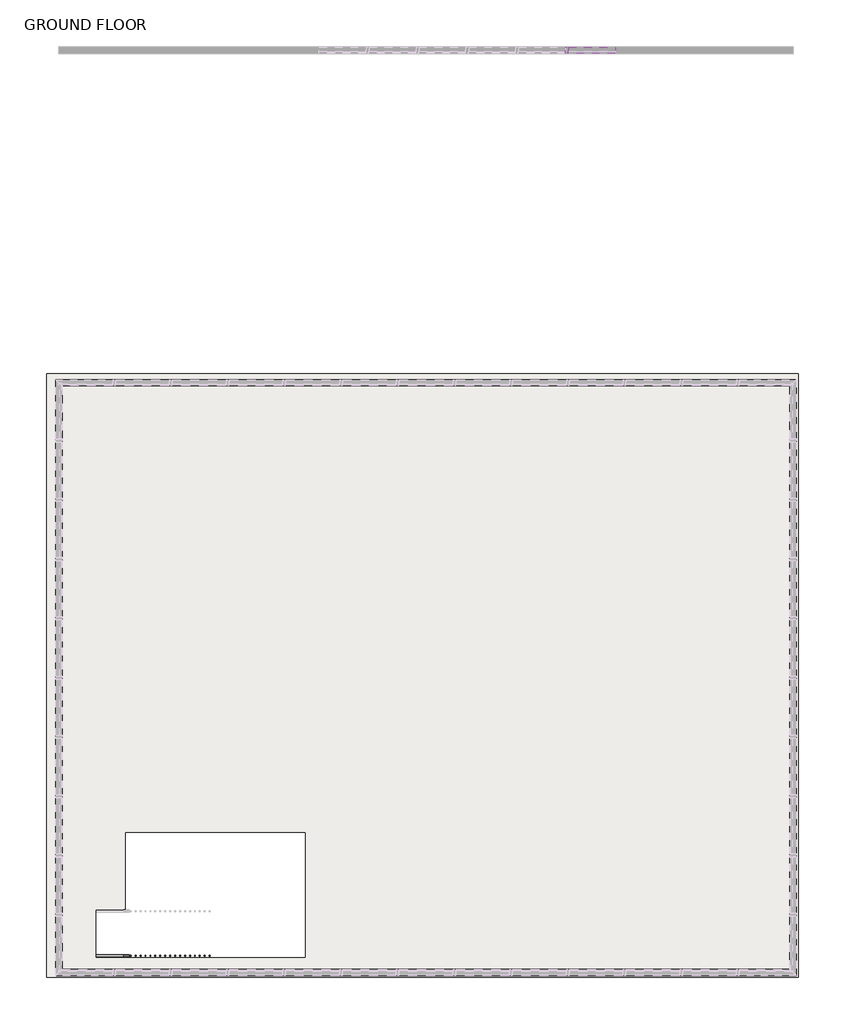
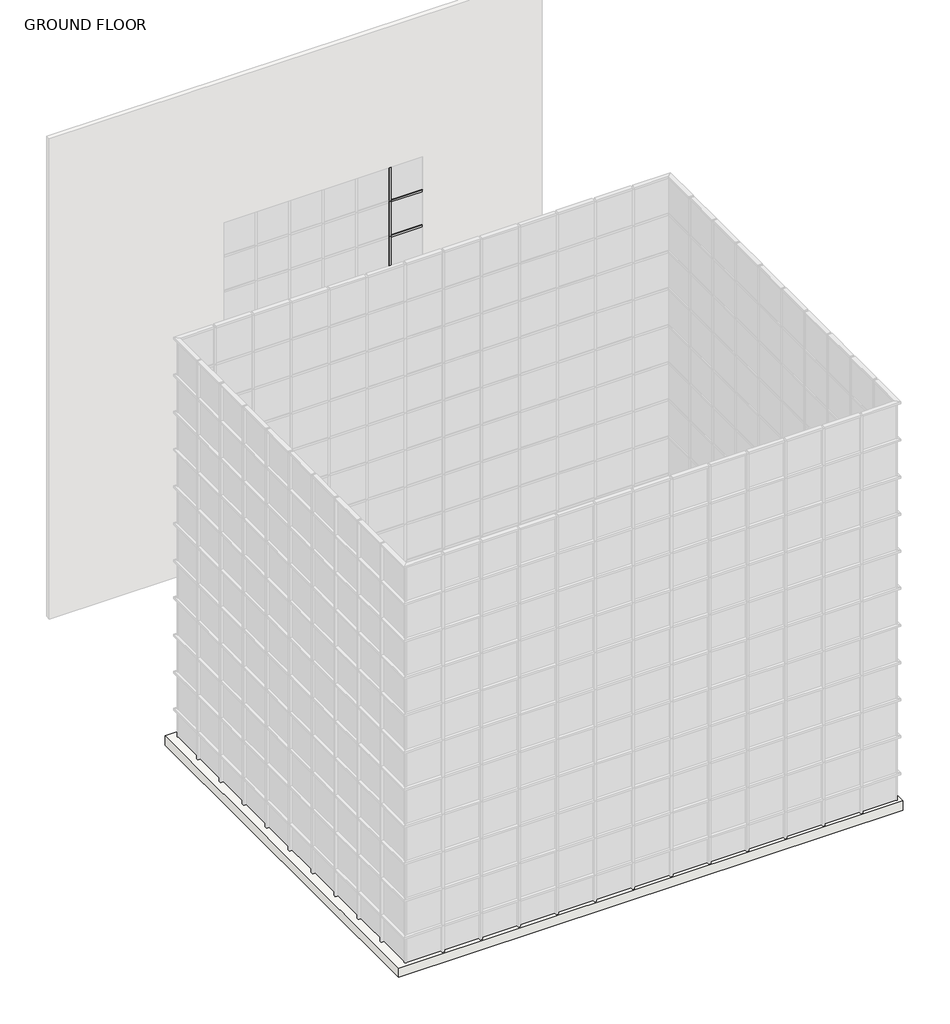
# One storey, part 15 of 16: 15 members, 1 railing, 1 slab.
"""IFC4 building model written with IfcOpenShell, lengths in millimetres."""

from ifc_helpers import new_model, si_unit, frame, origin, origin_with_axes, place, context, project, spatial, polyline, outline, extrude, faceted_brep, transform, mapped, element, save
from components import member_fdbefc00, member_3df3cfcf, member_368818a6

model = new_model("IFC4")

# Units and contexts
model_context = context("Model", 3, world=origin())
ifc_project = project(units=[si_unit("LENGTHUNIT", "METRE", prefix="MILLI")], contexts=[model_context])

# Site, building, storey
site = spatial("IfcSite", under=ifc_project)
building = spatial("IfcBuilding", under=site)
storey = spatial("IfcBuildingStorey", under=building, Name="GROUND FLOOR", Elevation=0.0)

# Members
placement = place(None, origin())
member_shape = member_fdbefc00(model_context)
element("IfcMember", 1, ObjectType="Rectangular Mullion : 2.5\" x 5\" rectangular", at=placement, inside=storey, context=model_context, shape_type="MappedRepresentation", body=[
    mapped(member_shape, transform((2306.4449607, 13200.7626438, 3045.6877023), x_axis=(0.0, 0.0, 1.0), y_axis=(0.0, -1.0, 0.0), z_axis=(1.0, 0.0, 0.0))),
])
element("IfcMember", 2, ObjectType="Rectangular Mullion : 2.5\" x 5\" rectangular", at=placement, inside=storey, context=model_context, shape_type="MappedRepresentation", body=[
    mapped(member_shape, transform((2306.4449607, 13200.7626438, 4181.5290519), x_axis=(0.0, 0.0, 1.0), y_axis=(0.0, -1.0, 0.0), z_axis=(1.0, 0.0, 0.0))),
])
element("IfcMember", 3, ObjectType="Rectangular Mullion : 2.5\" x 5\" rectangular", at=placement, inside=storey, context=model_context, shape_type="MappedRepresentation", body=[
    mapped(member_shape, transform((2306.4449607, 13200.7626438, 5317.3704015), x_axis=(0.0, 0.0, 1.0), y_axis=(0.0, -1.0, 0.0), z_axis=(1.0, 0.0, 0.0))),
])
element("IfcMember", 4, ObjectType="Rectangular Mullion : 2.5\" x 5\" rectangular", at=placement, inside=storey, context=model_context, shape_type="MappedRepresentation", body=[
    mapped(member_shape, transform((2306.4449607, 13200.7626438, 6453.2117511), x_axis=(0.0, 0.0, 1.0), y_axis=(0.0, -1.0, 0.0), z_axis=(1.0, 0.0, 0.0))),
])
element("IfcMember", 5, ObjectType="Rectangular Mullion : 2.5\" x 5\" rectangular", at=placement, inside=storey, context=model_context, shape_type="MappedRepresentation", body=[
    mapped(member_shape, transform((2306.4449607, 13200.7626438, 7589.0531007), x_axis=(0.0, 0.0, 1.0), y_axis=(0.0, -1.0, 0.0), z_axis=(1.0, 0.0, 0.0))),
])
element("IfcMember", 6, ObjectType="Rectangular Mullion : 2.5\" x 5\" rectangular", at=placement, inside=storey, context=model_context, shape_type="MappedRepresentation", body=[
    mapped(member_shape, transform((2306.4449607, 13200.7626438, 8724.8944503), x_axis=(0.0, 0.0, 1.0), y_axis=(0.0, -1.0, 0.0), z_axis=(1.0, 0.0, 0.0))),
])
element("IfcMember", 7, ObjectType="Rectangular Mullion : 2.5\" x 5\" rectangular", at=placement, inside=storey, context=model_context, shape_type="MappedRepresentation", body=[
    mapped(member_shape, transform((2306.4449607, 13200.7626438, 9860.7357999), x_axis=(0.0, 0.0, 1.0), y_axis=(0.0, -1.0, 0.0), z_axis=(1.0, 0.0, 0.0))),
])
member_2_shape = member_3df3cfcf(model_context)
element("IfcMember", 8, ObjectType="Rectangular Mullion : 2.5\" x 5\" rectangular", at=placement, inside=storey, context=model_context, shape_type="MappedRepresentation", body=[
    mapped(member_2_shape, transform((1314.3014531, 13200.7626438, 1941.5963527), x_axis=(1.0, 0.0, 0.0), y_axis=(0.0, -1.0, 0.0), z_axis=(0.0, 0.0, -1.0))),
])
member_3_shape = member_368818a6(model_context)
element("IfcMember", 9, ObjectType="Rectangular Mullion : 2.5\" x 5\" rectangular", at=placement, inside=storey, context=model_context, shape_type="MappedRepresentation", body=[
    mapped(member_3_shape, transform((1314.3014531, 13200.7626438, 3045.6877023), x_axis=(1.0, 0.0, 0.0), y_axis=(0.0, -1.0, 0.0), z_axis=(0.0, 0.0, -1.0))),
])
element("IfcMember", 10, ObjectType="Rectangular Mullion : 2.5\" x 5\" rectangular", at=placement, inside=storey, context=model_context, shape_type="MappedRepresentation", body=[
    mapped(member_3_shape, transform((1314.3014531, 13200.7626438, 4181.5290519), x_axis=(1.0, 0.0, 0.0), y_axis=(0.0, -1.0, 0.0), z_axis=(0.0, 0.0, -1.0))),
])
element("IfcMember", 11, ObjectType="Rectangular Mullion : 2.5\" x 5\" rectangular", at=placement, inside=storey, context=model_context, shape_type="MappedRepresentation", body=[
    mapped(member_3_shape, transform((1314.3014531, 13200.7626438, 5317.3704015), x_axis=(1.0, 0.0, 0.0), y_axis=(0.0, -1.0, 0.0), z_axis=(0.0, 0.0, -1.0))),
])
element("IfcMember", 12, ObjectType="Rectangular Mullion : 2.5\" x 5\" rectangular", at=placement, inside=storey, context=model_context, shape_type="MappedRepresentation", body=[
    mapped(member_3_shape, transform((1314.3014531, 13200.7626438, 6453.2117511), x_axis=(1.0, 0.0, 0.0), y_axis=(0.0, -1.0, 0.0), z_axis=(0.0, 0.0, -1.0))),
])
element("IfcMember", 13, ObjectType="Rectangular Mullion : 2.5\" x 5\" rectangular", at=placement, inside=storey, context=model_context, shape_type="MappedRepresentation", body=[
    mapped(member_3_shape, transform((1314.3014531, 13200.7626438, 7589.0531007), x_axis=(1.0, 0.0, 0.0), y_axis=(0.0, -1.0, 0.0), z_axis=(0.0, 0.0, -1.0))),
])
element("IfcMember", 14, ObjectType="Rectangular Mullion : 2.5\" x 5\" rectangular", at=placement, inside=storey, context=model_context, shape_type="MappedRepresentation", body=[
    mapped(member_3_shape, transform((1314.3014531, 13200.7626438, 8724.8944503), x_axis=(1.0, 0.0, 0.0), y_axis=(0.0, -1.0, 0.0), z_axis=(0.0, 0.0, -1.0))),
])
element("IfcMember", 15, ObjectType="Rectangular Mullion : 2.5\" x 5\" rectangular", at=placement, inside=storey, context=model_context, shape_type="MappedRepresentation", body=[
    mapped(member_2_shape, transform((1314.3014531, 13200.7626438, 9860.7357999), x_axis=(1.0, 0.0, 0.0), y_axis=(0.0, -1.0, 0.0), z_axis=(0.0, 0.0, -1.0))),
])

# Railing
element("IfcRailing", 16, ObjectType="Handrail - Rectangular", at=placement, inside=storey, context=model_context, shape_type="SolidModel", body=[
    faceted_brep([(-8362.2800418, -5370.1090076, 914.4), (-8362.2800418, -5370.1090076, 857.6038734), (-8362.2800418, -5420.9090076, 857.6038734), (-8362.2800418, -5420.9090076, 914.4), (-5009.4800418, -5370.1090076, 2590.8), (-4997.4877885, -5370.1090076, 2540.0), (-4997.4877885, -5420.9090076, 2540.0), (-5009.4800418, -5420.9090076, 2590.8), (-4120.4800418, -5370.1090076, 2590.8), (-4120.4800418, -5370.1090076, 2540.0), (-4069.6800418, -5420.9090076, 2540.0), (-4069.6800418, -5420.9090076, 2590.8), (-4120.4800418, -2917.1346494, 2590.8), (-4120.4800418, -2917.1346494, 2540.0), (-4069.6800418, -2866.3346494, 2540.0), (-4069.6800418, -2866.3346494, 2590.8), (-5009.4800418, -2917.1346494, 2590.8), (-5021.472295, -2917.1346494, 2540.0), (-5021.472295, -2866.3346494, 2540.0), (-5009.4800418, -2866.3346494, 2590.8), (-7752.6800418, -2917.1346494, 3962.4), (-7752.6800418, -2866.3346494, 3962.4), (-7752.6800418, -2866.3346494, 3905.6038734), (-7752.6800418, -2917.1346494, 3905.6038734)], [[[0, 1, 2, 3]], [[1, 0, 4, 5]], [[2, 1, 5, 6]], [[3, 2, 6, 7]], [[0, 3, 7, 4]], [[5, 4, 8, 9]], [[6, 5, 9, 10]], [[7, 6, 10, 11]], [[4, 7, 11, 8]], [[9, 8, 12, 13]], [[10, 9, 13, 14]], [[11, 10, 14, 15]], [[8, 11, 15, 12]], [[13, 12, 16, 17]], [[14, 13, 17, 18]], [[15, 14, 18, 19]], [[12, 15, 19, 16]], [[20, 21, 22, 23]], [[17, 16, 20, 23]], [[18, 17, 23, 22]], [[19, 18, 22, 21]], [[16, 19, 21, 20]]]),
    extrude(outline(polyline([(3859.5663734, -7660.6050418), (3001.9625, -7660.6050418), (2992.4375, -7641.5550418), (3850.0413734, -7641.5550418), (3859.5663734, -7660.6050418)])), frame((0.0, -2901.2596494, 0.0), z_axis=(0.0, 1.0, 0.0), x_axis=(0.0, 0.0, 1.0)), (0.0, 0.0, 1.0), 19.05),
    extrude(outline(polyline([(3808.7663734, -7559.0050418), (2951.1625, -7559.0050418), (2941.6375, -7539.9550418), (3799.2413734, -7539.9550418), (3808.7663734, -7559.0050418)])), frame((0.0, -2901.2596494, 0.0), z_axis=(0.0, 1.0, 0.0), x_axis=(0.0, 0.0, 1.0)), (0.0, 0.0, 1.0), 19.05),
    extrude(outline(polyline([(3757.9663734, -7457.4050418), (2900.3625, -7457.4050418), (2890.8375, -7438.3550418), (3748.4413734, -7438.3550418), (3757.9663734, -7457.4050418)])), frame((0.0, -2901.2596494, 0.0), z_axis=(0.0, 1.0, 0.0), x_axis=(0.0, 0.0, 1.0)), (0.0, 0.0, 1.0), 19.05),
    extrude(outline(polyline([(3707.1663734, -7355.8050418), (2849.5625, -7355.8050418), (2840.0375, -7336.7550418), (3697.6413734, -7336.7550418), (3707.1663734, -7355.8050418)])), frame((0.0, -2901.2596494, 0.0), z_axis=(0.0, 1.0, 0.0), x_axis=(0.0, 0.0, 1.0)), (0.0, 0.0, 1.0), 19.05),
    extrude(outline(polyline([(3656.3663734, -7254.2050418), (2798.7625, -7254.2050418), (2789.2375, -7235.1550418), (3646.8413734, -7235.1550418), (3656.3663734, -7254.2050418)])), frame((0.0, -2901.2596494, 0.0), z_axis=(0.0, 1.0, 0.0), x_axis=(0.0, 0.0, 1.0)), (0.0, 0.0, 1.0), 19.05),
    extrude(outline(polyline([(3605.5663734, -7152.6050418), (2747.9625, -7152.6050418), (2738.4375, -7133.5550418), (3596.0413734, -7133.5550418), (3605.5663734, -7152.6050418)])), frame((0.0, -2901.2596494, 0.0), z_axis=(0.0, 1.0, 0.0), x_axis=(0.0, 0.0, 1.0)), (0.0, 0.0, 1.0), 19.05),
    extrude(outline(polyline([(3554.7663734, -7051.0050418), (2697.1625, -7051.0050418), (2687.6375, -7031.9550418), (3545.2413734, -7031.9550418), (3554.7663734, -7051.0050418)])), frame((0.0, -2901.2596494, 0.0), z_axis=(0.0, 1.0, 0.0), x_axis=(0.0, 0.0, 1.0)), (0.0, 0.0, 1.0), 19.05),
    extrude(outline(polyline([(3503.9663734, -6949.4050418), (2646.3625, -6949.4050418), (2636.8375, -6930.3550418), (3494.4413734, -6930.3550418), (3503.9663734, -6949.4050418)])), frame((0.0, -2901.2596494, 0.0), z_axis=(0.0, 1.0, 0.0), x_axis=(0.0, 0.0, 1.0)), (0.0, 0.0, 1.0), 19.05),
    extrude(outline(polyline([(3453.1663734, -6847.8050418), (2595.5625, -6847.8050418), (2586.0375, -6828.7550418), (3443.6413734, -6828.7550418), (3453.1663734, -6847.8050418)])), frame((0.0, -2901.2596494, 0.0), z_axis=(0.0, 1.0, 0.0), x_axis=(0.0, 0.0, 1.0)), (0.0, 0.0, 1.0), 19.05),
    extrude(outline(polyline([(3402.3663734, -6746.2050418), (2544.7625, -6746.2050418), (2535.2375, -6727.1550418), (3392.8413734, -6727.1550418), (3402.3663734, -6746.2050418)])), frame((0.0, -2901.2596494, 0.0), z_axis=(0.0, 1.0, 0.0), x_axis=(0.0, 0.0, 1.0)), (0.0, 0.0, 1.0), 19.05),
    extrude(outline(polyline([(3351.5663734, -6644.6050418), (2493.9625, -6644.6050418), (2484.4375, -6625.5550418), (3342.0413734, -6625.5550418), (3351.5663734, -6644.6050418)])), frame((0.0, -2901.2596494, 0.0), z_axis=(0.0, 1.0, 0.0), x_axis=(0.0, 0.0, 1.0)), (0.0, 0.0, 1.0), 19.05),
    extrude(outline(polyline([(3300.7663734, -6543.0050418), (2443.1625, -6543.0050418), (2433.6375, -6523.9550418), (3291.2413734, -6523.9550418), (3300.7663734, -6543.0050418)])), frame((0.0, -2901.2596494, 0.0), z_axis=(0.0, 1.0, 0.0), x_axis=(0.0, 0.0, 1.0)), (0.0, 0.0, 1.0), 19.05),
    extrude(outline(polyline([(3249.9663734, -6441.4050418), (2392.3625, -6441.4050418), (2382.8375, -6422.3550418), (3240.4413734, -6422.3550418), (3249.9663734, -6441.4050418)])), frame((0.0, -2901.2596494, 0.0), z_axis=(0.0, 1.0, 0.0), x_axis=(0.0, 0.0, 1.0)), (0.0, 0.0, 1.0), 19.05),
    extrude(outline(polyline([(3199.1663734, -6339.8050418), (2341.5625, -6339.8050418), (2332.0375, -6320.7550418), (3189.6413734, -6320.7550418), (3199.1663734, -6339.8050418)])), frame((0.0, -2901.2596494, 0.0), z_axis=(0.0, 1.0, 0.0), x_axis=(0.0, 0.0, 1.0)), (0.0, 0.0, 1.0), 19.05),
    extrude(outline(polyline([(3148.3663734, -6238.2050418), (2290.7625, -6238.2050418), (2281.2375, -6219.1550418), (3138.8413734, -6219.1550418), (3148.3663734, -6238.2050418)])), frame((0.0, -2901.2596494, 0.0), z_axis=(0.0, 1.0, 0.0), x_axis=(0.0, 0.0, 1.0)), (0.0, 0.0, 1.0), 19.05),
    extrude(outline(polyline([(3097.5663734, -6136.6050418), (2239.9625, -6136.6050418), (2230.4375, -6117.5550418), (3088.0413734, -6117.5550418), (3097.5663734, -6136.6050418)])), frame((0.0, -2901.2596494, 0.0), z_axis=(0.0, 1.0, 0.0), x_axis=(0.0, 0.0, 1.0)), (0.0, 0.0, 1.0), 19.05),
    extrude(outline(polyline([(3046.7663734, -6035.0050418), (2189.1625, -6035.0050418), (2179.6375, -6015.9550418), (3037.2413734, -6015.9550418), (3046.7663734, -6035.0050418)])), frame((0.0, -2901.2596494, 0.0), z_axis=(0.0, 1.0, 0.0), x_axis=(0.0, 0.0, 1.0)), (0.0, 0.0, 1.0), 19.05),
    extrude(outline(polyline([(2995.9663734, -5933.4050418), (2138.3625, -5933.4050418), (2128.8375, -5914.3550418), (2986.4413734, -5914.3550418), (2995.9663734, -5933.4050418)])), frame((0.0, -2901.2596494, 0.0), z_axis=(0.0, 1.0, 0.0), x_axis=(0.0, 0.0, 1.0)), (0.0, 0.0, 1.0), 19.05),
    extrude(outline(polyline([(2945.1663734, -5831.8050418), (2087.5625, -5831.8050418), (2078.0375, -5812.7550418), (2935.6413734, -5812.7550418), (2945.1663734, -5831.8050418)])), frame((0.0, -2901.2596494, 0.0), z_axis=(0.0, 1.0, 0.0), x_axis=(0.0, 0.0, 1.0)), (0.0, 0.0, 1.0), 19.05),
    extrude(outline(polyline([(2894.3663734, -5730.2050418), (2036.7625, -5730.2050418), (2027.2375, -5711.1550418), (2884.8413734, -5711.1550418), (2894.3663734, -5730.2050418)])), frame((0.0, -2901.2596494, 0.0), z_axis=(0.0, 1.0, 0.0), x_axis=(0.0, 0.0, 1.0)), (0.0, 0.0, 1.0), 19.05),
    extrude(outline(polyline([(2843.5663734, -5628.6050418), (1985.9625, -5628.6050418), (1976.4375, -5609.5550418), (2834.0413734, -5609.5550418), (2843.5663734, -5628.6050418)])), frame((0.0, -2901.2596494, 0.0), z_axis=(0.0, 1.0, 0.0), x_axis=(0.0, 0.0, 1.0)), (0.0, 0.0, 1.0), 19.05),
    extrude(outline(polyline([(2792.7663734, -5527.0050418), (1935.1625, -5527.0050418), (1925.6375, -5507.9550418), (2783.2413734, -5507.9550418), (2792.7663734, -5527.0050418)])), frame((0.0, -2901.2596494, 0.0), z_axis=(0.0, 1.0, 0.0), x_axis=(0.0, 0.0, 1.0)), (0.0, 0.0, 1.0), 19.05),
    extrude(outline(polyline([(2741.9663734, -5425.4050418), (1884.3625, -5425.4050418), (1874.8375, -5406.3550418), (2732.4413734, -5406.3550418), (2741.9663734, -5425.4050418)])), frame((0.0, -2901.2596494, 0.0), z_axis=(0.0, 1.0, 0.0), x_axis=(0.0, 0.0, 1.0)), (0.0, 0.0, 1.0), 19.05),
    extrude(outline(polyline([(2691.1663734, -5323.8050418), (1833.5625, -5323.8050418), (1824.0375, -5304.7550418), (2681.6413734, -5304.7550418), (2691.1663734, -5323.8050418)])), frame((0.0, -2901.2596494, 0.0), z_axis=(0.0, 1.0, 0.0), x_axis=(0.0, 0.0, 1.0)), (0.0, 0.0, 1.0), 19.05),
    extrude(outline(polyline([(2640.3663734, -5222.2050418), (1782.7625, -5222.2050418), (1773.2375, -5203.1550418), (2630.8413734, -5203.1550418), (2640.3663734, -5222.2050418)])), frame((0.0, -2901.2596494, 0.0), z_axis=(0.0, 1.0, 0.0), x_axis=(0.0, 0.0, 1.0)), (0.0, 0.0, 1.0), 19.05),
    extrude(outline(polyline([(2589.5663734, -5120.6050418), (1731.9625, -5120.6050418), (1722.4375, -5101.5550418), (2580.0413734, -5101.5550418), (2589.5663734, -5120.6050418)])), frame((0.0, -2901.2596494, 0.0), z_axis=(0.0, 1.0, 0.0), x_axis=(0.0, 0.0, 1.0)), (0.0, 0.0, 1.0), 19.05),
    extrude(outline(polyline([(-4898.3550418, -2901.2596494), (-4917.4050418, -2901.2596494), (-4917.4050418, -2882.2096494), (-4898.3550418, -2882.2096494), (-4898.3550418, -2901.2596494)])), frame((0.0, 0.0, 1676.4), z_axis=(0.0, 0.0, 1.0), x_axis=(1.0, 0.0, 0.0)), (0.0, 0.0, 1.0), 863.6),
    extrude(outline(polyline([(-4796.7550418, -2901.2596494), (-4815.8050418, -2901.2596494), (-4815.8050418, -2882.2096494), (-4796.7550418, -2882.2096494), (-4796.7550418, -2901.2596494)])), frame((0.0, 0.0, 1676.4), z_axis=(0.0, 0.0, 1.0), x_axis=(1.0, 0.0, 0.0)), (0.0, 0.0, 1.0), 863.6),
    extrude(outline(polyline([(-4695.1550418, -2901.2596494), (-4714.2050418, -2901.2596494), (-4714.2050418, -2882.2096494), (-4695.1550418, -2882.2096494), (-4695.1550418, -2901.2596494)])), frame((0.0, 0.0, 1676.4), z_axis=(0.0, 0.0, 1.0), x_axis=(1.0, 0.0, 0.0)), (0.0, 0.0, 1.0), 863.6),
    extrude(outline(polyline([(-4593.5550418, -2901.2596494), (-4612.6050418, -2901.2596494), (-4612.6050418, -2882.2096494), (-4593.5550418, -2882.2096494), (-4593.5550418, -2901.2596494)])), frame((0.0, 0.0, 1676.4), z_axis=(0.0, 0.0, 1.0), x_axis=(1.0, 0.0, 0.0)), (0.0, 0.0, 1.0), 863.6),
    extrude(outline(polyline([(-4491.9550418, -2901.2596494), (-4511.0050418, -2901.2596494), (-4511.0050418, -2882.2096494), (-4491.9550418, -2882.2096494), (-4491.9550418, -2901.2596494)])), frame((0.0, 0.0, 1676.4), z_axis=(0.0, 0.0, 1.0), x_axis=(1.0, 0.0, 0.0)), (0.0, 0.0, 1.0), 863.6),
    extrude(outline(polyline([(-4390.3550418, -2901.2596494), (-4409.4050418, -2901.2596494), (-4409.4050418, -2882.2096494), (-4390.3550418, -2882.2096494), (-4390.3550418, -2901.2596494)])), frame((0.0, 0.0, 1676.4), z_axis=(0.0, 0.0, 1.0), x_axis=(1.0, 0.0, 0.0)), (0.0, 0.0, 1.0), 863.6),
    extrude(outline(polyline([(-4288.7550418, -2901.2596494), (-4307.8050418, -2901.2596494), (-4307.8050418, -2882.2096494), (-4288.7550418, -2882.2096494), (-4288.7550418, -2901.2596494)])), frame((0.0, 0.0, 1676.4), z_axis=(0.0, 0.0, 1.0), x_axis=(1.0, 0.0, 0.0)), (0.0, 0.0, 1.0), 863.6),
    extrude(outline(polyline([(-4187.1550418, -2901.2596494), (-4206.2050418, -2901.2596494), (-4206.2050418, -2882.2096494), (-4187.1550418, -2882.2096494), (-4187.1550418, -2901.2596494)])), frame((0.0, 0.0, 1676.4), z_axis=(0.0, 0.0, 1.0), x_axis=(1.0, 0.0, 0.0)), (0.0, 0.0, 1.0), 863.6),
    extrude(outline(polyline([(-4104.6050418, -2966.6340076), (-4104.6050418, -2947.5840076), (-4085.5550418, -2947.5840076), (-4085.5550418, -2966.6340076), (-4104.6050418, -2966.6340076)])), frame((0.0, 0.0, 1676.4), z_axis=(0.0, 0.0, 1.0), x_axis=(1.0, 0.0, 0.0)), (0.0, 0.0, 1.0), 863.6),
    extrude(outline(polyline([(-4104.6050418, -3068.2340076), (-4104.6050418, -3049.1840076), (-4085.5550418, -3049.1840076), (-4085.5550418, -3068.2340076), (-4104.6050418, -3068.2340076)])), frame((0.0, 0.0, 1676.4), z_axis=(0.0, 0.0, 1.0), x_axis=(1.0, 0.0, 0.0)), (0.0, 0.0, 1.0), 863.6),
    extrude(outline(polyline([(-4104.6050418, -3169.8340076), (-4104.6050418, -3150.7840076), (-4085.5550418, -3150.7840076), (-4085.5550418, -3169.8340076), (-4104.6050418, -3169.8340076)])), frame((0.0, 0.0, 1676.4), z_axis=(0.0, 0.0, 1.0), x_axis=(1.0, 0.0, 0.0)), (0.0, 0.0, 1.0), 863.6),
    extrude(outline(polyline([(-4104.6050418, -3271.4340076), (-4104.6050418, -3252.3840076), (-4085.5550418, -3252.3840076), (-4085.5550418, -3271.4340076), (-4104.6050418, -3271.4340076)])), frame((0.0, 0.0, 1676.4), z_axis=(0.0, 0.0, 1.0), x_axis=(1.0, 0.0, 0.0)), (0.0, 0.0, 1.0), 863.6),
    extrude(outline(polyline([(-4104.6050418, -3373.0340076), (-4104.6050418, -3353.9840076), (-4085.5550418, -3353.9840076), (-4085.5550418, -3373.0340076), (-4104.6050418, -3373.0340076)])), frame((0.0, 0.0, 1676.4), z_axis=(0.0, 0.0, 1.0), x_axis=(1.0, 0.0, 0.0)), (0.0, 0.0, 1.0), 863.6),
    extrude(outline(polyline([(-4104.6050418, -3474.6340076), (-4104.6050418, -3455.5840076), (-4085.5550418, -3455.5840076), (-4085.5550418, -3474.6340076), (-4104.6050418, -3474.6340076)])), frame((0.0, 0.0, 1676.4), z_axis=(0.0, 0.0, 1.0), x_axis=(1.0, 0.0, 0.0)), (0.0, 0.0, 1.0), 863.6),
    extrude(outline(polyline([(-4104.6050418, -3576.2340076), (-4104.6050418, -3557.1840076), (-4085.5550418, -3557.1840076), (-4085.5550418, -3576.2340076), (-4104.6050418, -3576.2340076)])), frame((0.0, 0.0, 1676.4), z_axis=(0.0, 0.0, 1.0), x_axis=(1.0, 0.0, 0.0)), (0.0, 0.0, 1.0), 863.6),
    extrude(outline(polyline([(-4104.6050418, -3677.8340076), (-4104.6050418, -3658.7840076), (-4085.5550418, -3658.7840076), (-4085.5550418, -3677.8340076), (-4104.6050418, -3677.8340076)])), frame((0.0, 0.0, 1676.4), z_axis=(0.0, 0.0, 1.0), x_axis=(1.0, 0.0, 0.0)), (0.0, 0.0, 1.0), 863.6),
    extrude(outline(polyline([(-4104.6050418, -3779.4340076), (-4104.6050418, -3760.3840076), (-4085.5550418, -3760.3840076), (-4085.5550418, -3779.4340076), (-4104.6050418, -3779.4340076)])), frame((0.0, 0.0, 1676.4), z_axis=(0.0, 0.0, 1.0), x_axis=(1.0, 0.0, 0.0)), (0.0, 0.0, 1.0), 863.6),
    extrude(outline(polyline([(-4104.6050418, -3881.0340076), (-4104.6050418, -3861.9840076), (-4085.5550418, -3861.9840076), (-4085.5550418, -3881.0340076), (-4104.6050418, -3881.0340076)])), frame((0.0, 0.0, 1676.4), z_axis=(0.0, 0.0, 1.0), x_axis=(1.0, 0.0, 0.0)), (0.0, 0.0, 1.0), 863.6),
    extrude(outline(polyline([(-4104.6050418, -3982.6340076), (-4104.6050418, -3963.5840076), (-4085.5550418, -3963.5840076), (-4085.5550418, -3982.6340076), (-4104.6050418, -3982.6340076)])), frame((0.0, 0.0, 1676.4), z_axis=(0.0, 0.0, 1.0), x_axis=(1.0, 0.0, 0.0)), (0.0, 0.0, 1.0), 863.6),
    extrude(outline(polyline([(-4104.6050418, -4084.2340076), (-4104.6050418, -4065.1840076), (-4085.5550418, -4065.1840076), (-4085.5550418, -4084.2340076), (-4104.6050418, -4084.2340076)])), frame((0.0, 0.0, 1676.4), z_axis=(0.0, 0.0, 1.0), x_axis=(1.0, 0.0, 0.0)), (0.0, 0.0, 1.0), 863.6),
    extrude(outline(polyline([(-4104.6050418, -4185.8340076), (-4104.6050418, -4166.7840076), (-4085.5550418, -4166.7840076), (-4085.5550418, -4185.8340076), (-4104.6050418, -4185.8340076)])), frame((0.0, 0.0, 1676.4), z_axis=(0.0, 0.0, 1.0), x_axis=(1.0, 0.0, 0.0)), (0.0, 0.0, 1.0), 863.6),
    extrude(outline(polyline([(-4104.6050418, -4287.4340076), (-4104.6050418, -4268.3840076), (-4085.5550418, -4268.3840076), (-4085.5550418, -4287.4340076), (-4104.6050418, -4287.4340076)])), frame((0.0, 0.0, 1676.4), z_axis=(0.0, 0.0, 1.0), x_axis=(1.0, 0.0, 0.0)), (0.0, 0.0, 1.0), 863.6),
    extrude(outline(polyline([(-4104.6050418, -4389.0340076), (-4104.6050418, -4369.9840076), (-4085.5550418, -4369.9840076), (-4085.5550418, -4389.0340076), (-4104.6050418, -4389.0340076)])), frame((0.0, 0.0, 1676.4), z_axis=(0.0, 0.0, 1.0), x_axis=(1.0, 0.0, 0.0)), (0.0, 0.0, 1.0), 863.6),
    extrude(outline(polyline([(-4104.6050418, -4490.6340076), (-4104.6050418, -4471.5840076), (-4085.5550418, -4471.5840076), (-4085.5550418, -4490.6340076), (-4104.6050418, -4490.6340076)])), frame((0.0, 0.0, 1676.4), z_axis=(0.0, 0.0, 1.0), x_axis=(1.0, 0.0, 0.0)), (0.0, 0.0, 1.0), 863.6),
    extrude(outline(polyline([(-4104.6050418, -4592.2340076), (-4104.6050418, -4573.1840076), (-4085.5550418, -4573.1840076), (-4085.5550418, -4592.2340076), (-4104.6050418, -4592.2340076)])), frame((0.0, 0.0, 1676.4), z_axis=(0.0, 0.0, 1.0), x_axis=(1.0, 0.0, 0.0)), (0.0, 0.0, 1.0), 863.6),
    extrude(outline(polyline([(-4104.6050418, -4693.8340076), (-4104.6050418, -4674.7840076), (-4085.5550418, -4674.7840076), (-4085.5550418, -4693.8340076), (-4104.6050418, -4693.8340076)])), frame((0.0, 0.0, 1676.4), z_axis=(0.0, 0.0, 1.0), x_axis=(1.0, 0.0, 0.0)), (0.0, 0.0, 1.0), 863.6),
    extrude(outline(polyline([(-4104.6050418, -4795.4340076), (-4104.6050418, -4776.3840076), (-4085.5550418, -4776.3840076), (-4085.5550418, -4795.4340076), (-4104.6050418, -4795.4340076)])), frame((0.0, 0.0, 1676.4), z_axis=(0.0, 0.0, 1.0), x_axis=(1.0, 0.0, 0.0)), (0.0, 0.0, 1.0), 863.6),
    extrude(outline(polyline([(-4104.6050418, -4897.0340076), (-4104.6050418, -4877.9840076), (-4085.5550418, -4877.9840076), (-4085.5550418, -4897.0340076), (-4104.6050418, -4897.0340076)])), frame((0.0, 0.0, 1676.4), z_axis=(0.0, 0.0, 1.0), x_axis=(1.0, 0.0, 0.0)), (0.0, 0.0, 1.0), 863.6),
    extrude(outline(polyline([(-4104.6050418, -4998.6340076), (-4104.6050418, -4979.5840076), (-4085.5550418, -4979.5840076), (-4085.5550418, -4998.6340076), (-4104.6050418, -4998.6340076)])), frame((0.0, 0.0, 1676.4), z_axis=(0.0, 0.0, 1.0), x_axis=(1.0, 0.0, 0.0)), (0.0, 0.0, 1.0), 863.6),
    extrude(outline(polyline([(-4104.6050418, -5100.2340076), (-4104.6050418, -5081.1840076), (-4085.5550418, -5081.1840076), (-4085.5550418, -5100.2340076), (-4104.6050418, -5100.2340076)])), frame((0.0, 0.0, 1676.4), z_axis=(0.0, 0.0, 1.0), x_axis=(1.0, 0.0, 0.0)), (0.0, 0.0, 1.0), 863.6),
    extrude(outline(polyline([(-4104.6050418, -5201.8340076), (-4104.6050418, -5182.7840076), (-4085.5550418, -5182.7840076), (-4085.5550418, -5201.8340076), (-4104.6050418, -5201.8340076)])), frame((0.0, 0.0, 1676.4), z_axis=(0.0, 0.0, 1.0), x_axis=(1.0, 0.0, 0.0)), (0.0, 0.0, 1.0), 863.6),
    extrude(outline(polyline([(-4104.6050418, -5303.4340076), (-4104.6050418, -5284.3840076), (-4085.5550418, -5284.3840076), (-4085.5550418, -5303.4340076), (-4104.6050418, -5303.4340076)])), frame((0.0, 0.0, 1676.4), z_axis=(0.0, 0.0, 1.0), x_axis=(1.0, 0.0, 0.0)), (0.0, 0.0, 1.0), 863.6),
    extrude(outline(polyline([(-4206.2050418, -5385.9840076), (-4187.1550418, -5385.9840076), (-4187.1550418, -5405.0340076), (-4206.2050418, -5405.0340076), (-4206.2050418, -5385.9840076)])), frame((0.0, 0.0, 1676.4), z_axis=(0.0, 0.0, 1.0), x_axis=(1.0, 0.0, 0.0)), (0.0, 0.0, 1.0), 863.6),
    extrude(outline(polyline([(-4307.8050418, -5385.9840076), (-4288.7550418, -5385.9840076), (-4288.7550418, -5405.0340076), (-4307.8050418, -5405.0340076), (-4307.8050418, -5385.9840076)])), frame((0.0, 0.0, 1676.4), z_axis=(0.0, 0.0, 1.0), x_axis=(1.0, 0.0, 0.0)), (0.0, 0.0, 1.0), 863.6),
    extrude(outline(polyline([(-4409.4050418, -5385.9840076), (-4390.3550418, -5385.9840076), (-4390.3550418, -5405.0340076), (-4409.4050418, -5405.0340076), (-4409.4050418, -5385.9840076)])), frame((0.0, 0.0, 1676.4), z_axis=(0.0, 0.0, 1.0), x_axis=(1.0, 0.0, 0.0)), (0.0, 0.0, 1.0), 863.6),
    extrude(outline(polyline([(-4511.0050418, -5385.9840076), (-4491.9550418, -5385.9840076), (-4491.9550418, -5405.0340076), (-4511.0050418, -5405.0340076), (-4511.0050418, -5385.9840076)])), frame((0.0, 0.0, 1676.4), z_axis=(0.0, 0.0, 1.0), x_axis=(1.0, 0.0, 0.0)), (0.0, 0.0, 1.0), 863.6),
    extrude(outline(polyline([(-4612.6050418, -5385.9840076), (-4593.5550418, -5385.9840076), (-4593.5550418, -5405.0340076), (-4612.6050418, -5405.0340076), (-4612.6050418, -5385.9840076)])), frame((0.0, 0.0, 1676.4), z_axis=(0.0, 0.0, 1.0), x_axis=(1.0, 0.0, 0.0)), (0.0, 0.0, 1.0), 863.6),
    extrude(outline(polyline([(-4714.2050418, -5385.9840076), (-4695.1550418, -5385.9840076), (-4695.1550418, -5405.0340076), (-4714.2050418, -5405.0340076), (-4714.2050418, -5385.9840076)])), frame((0.0, 0.0, 1676.4), z_axis=(0.0, 0.0, 1.0), x_axis=(1.0, 0.0, 0.0)), (0.0, 0.0, 1.0), 863.6),
    extrude(outline(polyline([(-4815.8050418, -5385.9840076), (-4796.7550418, -5385.9840076), (-4796.7550418, -5405.0340076), (-4815.8050418, -5405.0340076), (-4815.8050418, -5385.9840076)])), frame((0.0, 0.0, 1676.4), z_axis=(0.0, 0.0, 1.0), x_axis=(1.0, 0.0, 0.0)), (0.0, 0.0, 1.0), 863.6),
    extrude(outline(polyline([(-4917.4050418, -5385.9840076), (-4898.3550418, -5385.9840076), (-4898.3550418, -5405.0340076), (-4917.4050418, -5405.0340076), (-4917.4050418, -5385.9840076)])), frame((0.0, 0.0, 1676.4), z_axis=(0.0, 0.0, 1.0), x_axis=(1.0, 0.0, 0.0)), (0.0, 0.0, 1.0), 863.6),
    extrude(outline(polyline([(2478.4413734, -5120.6050418), (1620.8375, -5120.6050418), (1630.3625, -5101.5550418), (2487.9663734, -5101.5550418), (2478.4413734, -5120.6050418)])), frame((0.0, -5405.0340076, 0.0), z_axis=(0.0, 1.0, 0.0), x_axis=(0.0, 0.0, 1.0)), (0.0, 0.0, 1.0), 19.05),
    extrude(outline(polyline([(2427.6413734, -5222.2050418), (1570.0375, -5222.2050418), (1579.5625, -5203.1550418), (2437.1663734, -5203.1550418), (2427.6413734, -5222.2050418)])), frame((0.0, -5405.0340076, 0.0), z_axis=(0.0, 1.0, 0.0), x_axis=(0.0, 0.0, 1.0)), (0.0, 0.0, 1.0), 19.05),
    extrude(outline(polyline([(2376.8413734, -5323.8050418), (1519.2375, -5323.8050418), (1528.7625, -5304.7550418), (2386.3663734, -5304.7550418), (2376.8413734, -5323.8050418)])), frame((0.0, -5405.0340076, 0.0), z_axis=(0.0, 1.0, 0.0), x_axis=(0.0, 0.0, 1.0)), (0.0, 0.0, 1.0), 19.05),
    extrude(outline(polyline([(2326.0413734, -5425.4050418), (1468.4375, -5425.4050418), (1477.9625, -5406.3550418), (2335.5663734, -5406.3550418), (2326.0413734, -5425.4050418)])), frame((0.0, -5405.0340076, 0.0), z_axis=(0.0, 1.0, 0.0), x_axis=(0.0, 0.0, 1.0)), (0.0, 0.0, 1.0), 19.05),
    extrude(outline(polyline([(2275.2413734, -5527.0050418), (1417.6375, -5527.0050418), (1427.1625, -5507.9550418), (2284.7663734, -5507.9550418), (2275.2413734, -5527.0050418)])), frame((0.0, -5405.0340076, 0.0), z_axis=(0.0, 1.0, 0.0), x_axis=(0.0, 0.0, 1.0)), (0.0, 0.0, 1.0), 19.05),
    extrude(outline(polyline([(2224.4413734, -5628.6050418), (1366.8375, -5628.6050418), (1376.3625, -5609.5550418), (2233.9663734, -5609.5550418), (2224.4413734, -5628.6050418)])), frame((0.0, -5405.0340076, 0.0), z_axis=(0.0, 1.0, 0.0), x_axis=(0.0, 0.0, 1.0)), (0.0, 0.0, 1.0), 19.05),
    extrude(outline(polyline([(2173.6413734, -5730.2050418), (1316.0375, -5730.2050418), (1325.5625, -5711.1550418), (2183.1663734, -5711.1550418), (2173.6413734, -5730.2050418)])), frame((0.0, -5405.0340076, 0.0), z_axis=(0.0, 1.0, 0.0), x_axis=(0.0, 0.0, 1.0)), (0.0, 0.0, 1.0), 19.05),
    extrude(outline(polyline([(2122.8413734, -5831.8050418), (1265.2375, -5831.8050418), (1274.7625, -5812.7550418), (2132.3663734, -5812.7550418), (2122.8413734, -5831.8050418)])), frame((0.0, -5405.0340076, 0.0), z_axis=(0.0, 1.0, 0.0), x_axis=(0.0, 0.0, 1.0)), (0.0, 0.0, 1.0), 19.05),
    extrude(outline(polyline([(2072.0413734, -5933.4050418), (1214.4375, -5933.4050418), (1223.9625, -5914.3550418), (2081.5663734, -5914.3550418), (2072.0413734, -5933.4050418)])), frame((0.0, -5405.0340076, 0.0), z_axis=(0.0, 1.0, 0.0), x_axis=(0.0, 0.0, 1.0)), (0.0, 0.0, 1.0), 19.05),
    extrude(outline(polyline([(2021.2413734, -6035.0050418), (1163.6375, -6035.0050418), (1173.1625, -6015.9550418), (2030.7663734, -6015.9550418), (2021.2413734, -6035.0050418)])), frame((0.0, -5405.0340076, 0.0), z_axis=(0.0, 1.0, 0.0), x_axis=(0.0, 0.0, 1.0)), (0.0, 0.0, 1.0), 19.05),
    extrude(outline(polyline([(1970.4413734, -6136.6050418), (1112.8375, -6136.6050418), (1122.3625, -6117.5550418), (1979.9663734, -6117.5550418), (1970.4413734, -6136.6050418)])), frame((0.0, -5405.0340076, 0.0), z_axis=(0.0, 1.0, 0.0), x_axis=(0.0, 0.0, 1.0)), (0.0, 0.0, 1.0), 19.05),
    extrude(outline(polyline([(1919.6413734, -6238.2050418), (1062.0375, -6238.2050418), (1071.5625, -6219.1550418), (1929.1663734, -6219.1550418), (1919.6413734, -6238.2050418)])), frame((0.0, -5405.0340076, 0.0), z_axis=(0.0, 1.0, 0.0), x_axis=(0.0, 0.0, 1.0)), (0.0, 0.0, 1.0), 19.05),
    extrude(outline(polyline([(1868.8413734, -6339.8050418), (1011.2375, -6339.8050418), (1020.7625, -6320.7550418), (1878.3663734, -6320.7550418), (1868.8413734, -6339.8050418)])), frame((0.0, -5405.0340076, 0.0), z_axis=(0.0, 1.0, 0.0), x_axis=(0.0, 0.0, 1.0)), (0.0, 0.0, 1.0), 19.05),
    extrude(outline(polyline([(1818.0413734, -6441.4050418), (960.4375, -6441.4050418), (969.9625, -6422.3550418), (1827.5663734, -6422.3550418), (1818.0413734, -6441.4050418)])), frame((0.0, -5405.0340076, 0.0), z_axis=(0.0, 1.0, 0.0), x_axis=(0.0, 0.0, 1.0)), (0.0, 0.0, 1.0), 19.05),
    extrude(outline(polyline([(1767.2413734, -6543.0050418), (909.6375, -6543.0050418), (919.1625, -6523.9550418), (1776.7663734, -6523.9550418), (1767.2413734, -6543.0050418)])), frame((0.0, -5405.0340076, 0.0), z_axis=(0.0, 1.0, 0.0), x_axis=(0.0, 0.0, 1.0)), (0.0, 0.0, 1.0), 19.05),
    extrude(outline(polyline([(1716.4413734, -6644.6050418), (858.8375, -6644.6050418), (868.3625, -6625.5550418), (1725.9663734, -6625.5550418), (1716.4413734, -6644.6050418)])), frame((0.0, -5405.0340076, 0.0), z_axis=(0.0, 1.0, 0.0), x_axis=(0.0, 0.0, 1.0)), (0.0, 0.0, 1.0), 19.05),
    extrude(outline(polyline([(1665.6413734, -6746.2050418), (808.0375, -6746.2050418), (817.5625, -6727.1550418), (1675.1663734, -6727.1550418), (1665.6413734, -6746.2050418)])), frame((0.0, -5405.0340076, 0.0), z_axis=(0.0, 1.0, 0.0), x_axis=(0.0, 0.0, 1.0)), (0.0, 0.0, 1.0), 19.05),
    extrude(outline(polyline([(1614.8413734, -6847.8050418), (757.2375, -6847.8050418), (766.7625, -6828.7550418), (1624.3663734, -6828.7550418), (1614.8413734, -6847.8050418)])), frame((0.0, -5405.0340076, 0.0), z_axis=(0.0, 1.0, 0.0), x_axis=(0.0, 0.0, 1.0)), (0.0, 0.0, 1.0), 19.05),
    extrude(outline(polyline([(1564.0413734, -6949.4050418), (706.4375, -6949.4050418), (715.9625, -6930.3550418), (1573.5663734, -6930.3550418), (1564.0413734, -6949.4050418)])), frame((0.0, -5405.0340076, 0.0), z_axis=(0.0, 1.0, 0.0), x_axis=(0.0, 0.0, 1.0)), (0.0, 0.0, 1.0), 19.05),
    extrude(outline(polyline([(1513.2413734, -7051.0050418), (655.6375, -7051.0050418), (665.1625, -7031.9550418), (1522.7663734, -7031.9550418), (1513.2413734, -7051.0050418)])), frame((0.0, -5405.0340076, 0.0), z_axis=(0.0, 1.0, 0.0), x_axis=(0.0, 0.0, 1.0)), (0.0, 0.0, 1.0), 19.05),
    extrude(outline(polyline([(1462.4413734, -7152.6050418), (604.8375, -7152.6050418), (614.3625, -7133.5550418), (1471.9663734, -7133.5550418), (1462.4413734, -7152.6050418)])), frame((0.0, -5405.0340076, 0.0), z_axis=(0.0, 1.0, 0.0), x_axis=(0.0, 0.0, 1.0)), (0.0, 0.0, 1.0), 19.05),
    extrude(outline(polyline([(1411.6413734, -7254.2050418), (554.0375, -7254.2050418), (563.5625, -7235.1550418), (1421.1663734, -7235.1550418), (1411.6413734, -7254.2050418)])), frame((0.0, -5405.0340076, 0.0), z_axis=(0.0, 1.0, 0.0), x_axis=(0.0, 0.0, 1.0)), (0.0, 0.0, 1.0), 19.05),
    extrude(outline(polyline([(1360.8413734, -7355.8050418), (503.2375, -7355.8050418), (512.7625, -7336.7550418), (1370.3663734, -7336.7550418), (1360.8413734, -7355.8050418)])), frame((0.0, -5405.0340076, 0.0), z_axis=(0.0, 1.0, 0.0), x_axis=(0.0, 0.0, 1.0)), (0.0, 0.0, 1.0), 19.05),
    extrude(outline(polyline([(1310.0413734, -7457.4050418), (452.4375, -7457.4050418), (461.9625, -7438.3550418), (1319.5663734, -7438.3550418), (1310.0413734, -7457.4050418)])), frame((0.0, -5405.0340076, 0.0), z_axis=(0.0, 1.0, 0.0), x_axis=(0.0, 0.0, 1.0)), (0.0, 0.0, 1.0), 19.05),
    extrude(outline(polyline([(1259.2413734, -7559.0050418), (401.6375, -7559.0050418), (411.1625, -7539.9550418), (1268.7663734, -7539.9550418), (1259.2413734, -7559.0050418)])), frame((0.0, -5405.0340076, 0.0), z_axis=(0.0, 1.0, 0.0), x_axis=(0.0, 0.0, 1.0)), (0.0, 0.0, 1.0), 19.05),
    extrude(outline(polyline([(1208.4413734, -7660.6050418), (350.8375, -7660.6050418), (360.3625, -7641.5550418), (1217.9663734, -7641.5550418), (1208.4413734, -7660.6050418)])), frame((0.0, -5405.0340076, 0.0), z_axis=(0.0, 1.0, 0.0), x_axis=(0.0, 0.0, 1.0)), (0.0, 0.0, 1.0), 19.05),
    extrude(outline(polyline([(1157.6413734, -7762.2050418), (300.0375, -7762.2050418), (309.5625, -7743.1550418), (1167.1663734, -7743.1550418), (1157.6413734, -7762.2050418)])), frame((0.0, -5405.0340076, 0.0), z_axis=(0.0, 1.0, 0.0), x_axis=(0.0, 0.0, 1.0)), (0.0, 0.0, 1.0), 19.05),
    extrude(outline(polyline([(1106.8413734, -7863.8050418), (249.2375, -7863.8050418), (258.7625, -7844.7550418), (1116.3663734, -7844.7550418), (1106.8413734, -7863.8050418)])), frame((0.0, -5405.0340076, 0.0), z_axis=(0.0, 1.0, 0.0), x_axis=(0.0, 0.0, 1.0)), (0.0, 0.0, 1.0), 19.05),
    extrude(outline(polyline([(1056.0413734, -7965.4050418), (198.4375, -7965.4050418), (207.9625, -7946.3550418), (1065.5663734, -7946.3550418), (1056.0413734, -7965.4050418)])), frame((0.0, -5405.0340076, 0.0), z_axis=(0.0, 1.0, 0.0), x_axis=(0.0, 0.0, 1.0)), (0.0, 0.0, 1.0), 19.05),
    extrude(outline(polyline([(1005.2413734, -8067.0050418), (147.6375, -8067.0050418), (157.1625, -8047.9550418), (1014.7663734, -8047.9550418), (1005.2413734, -8067.0050418)])), frame((0.0, -5405.0340076, 0.0), z_axis=(0.0, 1.0, 0.0), x_axis=(0.0, 0.0, 1.0)), (0.0, 0.0, 1.0), 19.05),
    extrude(outline(polyline([(954.4413734, -8168.6050418), (96.8375, -8168.6050418), (106.3625, -8149.5550418), (963.9663734, -8149.5550418), (954.4413734, -8168.6050418)])), frame((0.0, -5405.0340076, 0.0), z_axis=(0.0, 1.0, 0.0), x_axis=(0.0, 0.0, 1.0)), (0.0, 0.0, 1.0), 19.05),
    extrude(outline(polyline([(903.6413734, -8270.2050418), (46.0375, -8270.2050418), (55.5625, -8251.1550418), (913.1663734, -8251.1550418), (903.6413734, -8270.2050418)])), frame((0.0, -5405.0340076, 0.0), z_axis=(0.0, 1.0, 0.0), x_axis=(0.0, 0.0, 1.0)), (0.0, 0.0, 1.0), 19.05),
    extrude(outline(polyline([(-4999.9550418, -2901.2596494), (-5019.0050418, -2901.2596494), (-5019.0050418, -2882.2096494), (-4999.9550418, -2882.2096494), (-4999.9550418, -2901.2596494)])), frame((0.0, 0.0, 1676.4), z_axis=(0.0, 0.0, 1.0), x_axis=(1.0, 0.0, 0.0)), (0.0, 0.0, 1.0), 863.6),
    extrude(outline(polyline([(-4104.6050418, -2901.2596494), (-4104.6050418, -2882.2096494), (-4085.5550418, -2882.2096494), (-4085.5550418, -2901.2596494), (-4104.6050418, -2901.2596494)])), frame((0.0, 0.0, 1676.4), z_axis=(0.0, 0.0, 1.0), x_axis=(1.0, 0.0, 0.0)), (0.0, 0.0, 1.0), 863.6),
    extrude(outline(polyline([(-4104.6050418, -5385.9840076), (-4085.5550418, -5385.9840076), (-4085.5550418, -5405.0340076), (-4104.6050418, -5405.0340076), (-4104.6050418, -5385.9840076)])), frame((0.0, 0.0, 1676.4), z_axis=(0.0, 0.0, 1.0), x_axis=(1.0, 0.0, 0.0)), (0.0, 0.0, 1.0), 863.6),
    extrude(outline(polyline([(2529.2413734, -5019.0050418), (1671.6375, -5019.0050418), (1681.1625, -4999.9550418), (2538.7663734, -4999.9550418), (2529.2413734, -5019.0050418)])), frame((0.0, -5405.0340076, 0.0), z_axis=(0.0, 1.0, 0.0), x_axis=(0.0, 0.0, 1.0)), (0.0, 0.0, 1.0), 19.05),
    extrude(outline(polyline([(3905.6038734, -7752.6800418), (3048.0, -7752.6800418), (3038.475, -7733.6300418), (3896.0788734, -7733.6300418), (3905.6038734, -7752.6800418)])), frame((0.0, -2901.2596494, 0.0), z_axis=(0.0, 1.0, 0.0), x_axis=(0.0, 0.0, 1.0)), (0.0, 0.0, 1.0), 19.05),
    extrude(outline(polyline([(857.6038734, -8362.2800418), (0.0, -8362.2800418), (9.525, -8343.2300418), (867.1288734, -8343.2300418), (857.6038734, -8362.2800418)])), frame((0.0, -5405.0340076, 0.0), z_axis=(0.0, 1.0, 0.0), x_axis=(0.0, 0.0, 1.0)), (0.0, 0.0, 1.0), 19.05),
])

# Slab
element("IfcSlab", 17, ObjectType="Generic - 12\"", at=placement, inside=storey, context=model_context, shape_type="SweptSolid", body=[
    extrude(outline(polyline([(6064.2982466, 6554.3761968), (6064.2982466, -5840.8238032), (-9378.9017534, -5840.8238032), (-9378.9017534, 6554.3761968), (6064.2982466, 6554.3761968)]), holes=[polyline([(-7752.6800418, -2866.3346494), (-7752.6800418, -4455.7090076), (-8362.2800418, -4455.7090076), (-8362.2800418, -5420.9090076), (-4069.6800418, -5420.9090076), (-4069.6800418, -2866.3346494), (-7752.6800418, -2866.3346494)])]), origin_with_axes(), (0.0, 0.0, 1.0), 304.8),
])

save(model, "model.ifc")

# Revit data of these elements
# Type "Rectangular Mullion : 2.5\" x 5\" rectangular"
#   built-in parameter 1007304 = 0.416667 (stored number, unit not read)
#   built-in parameter 1007301 = 0.104167 (stored number, unit not read)
#   built-in parameter 1007300 = 0.104167 (stored number, unit not read)
# Type "Handrail - Rectangular"
#   Assembly Code = "C2010400"
#   built-in parameter 1008612 = 0.0416667 (stored number, unit not read)
#   built-in parameter 1008611 = 0.0416667 (stored number, unit not read)
#   built-in parameter 1008609 = 0.333333 (stored number, unit not read)
#   built-in parameter 1008604 = 0.166667 (stored number, unit not read)
#   built-in parameter 1008603 = 0.166667 (stored number, unit not read)
#   Railing Height = 3' - 0"
#   built-in parameter 1008630 = 2
#   built-in parameter 1008610 = 2
#   built-in parameter 1008618 = Baluster - Square : 3/4"
# Type "Generic - 12\""
#   Assembly Code = "B1010"
#   Function = 0
#   Layers, outside or top first: 1' - 0" no material (function 1)
# Elements 1, 2, 3, 4, 5, 6, 7, 8, 9, 10, 11, 12, 13, 14, 15 (IfcMember, "Rectangular Mullion : 2.5\" x 5\" rectangular")
#   Phase Created = New Construction
#   Materials on its faces: "Aluminum"
# Element 16 (IfcRailing, "Handrail - Rectangular")
#   Phase Created = New Construction
# Element 17 (IfcSlab, "Generic - 12\"")
#   Height Offset From Level = 1' - 0"
#   Phase Created = New Construction
#   Materials on its faces: "Default Floor"
# Materials
#   "Aluminum": class "Metal", colour RGB 247 247 247, transparency 0, Description = "Aluminum 6061", Cost = 0
#   "Default Floor": colour RGB 128 128 128, transparency 0, Cost = 0
